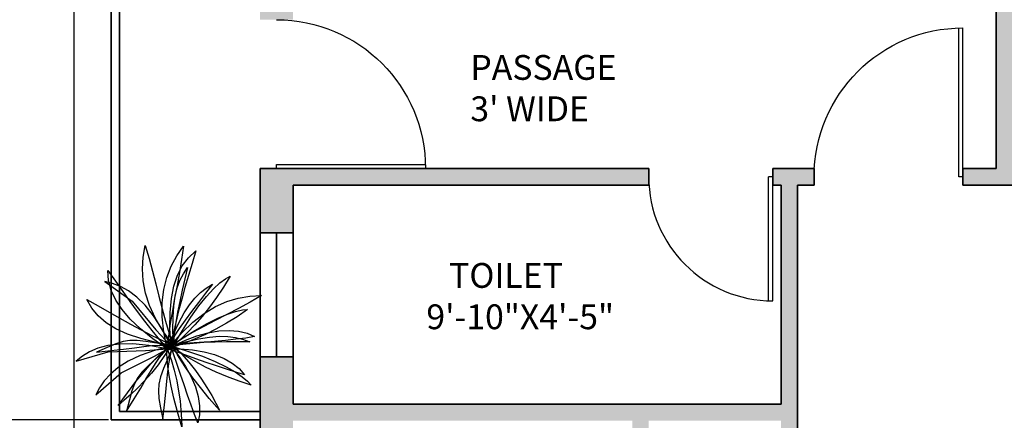
# Model space of a CAD drawing. Units: inches. Extents: x 1566 to 2546, y 1087 to 2705.
# Tile 19 of 27: x 2040 to 2278, y 1529 to 1625. Entities that reach past the tile are written whole.
import ezdxf

# ---------------------------------------------------------------- set-up
doc = ezdxf.new("R2010")
doc.units = ezdxf.units.IN
for name, color, linetype, lineweight in [('A-ANNO-DIMS', 2, 'Continuous', 18), ('A-AREA-IDEN', 7, 'Continuous', 18), ('A-DOOR', 4, 'Continuous', 25), ('A-WALL', 7, 'Continuous', 35), ('A-WALL-PATT', 8, 'Continuous', 13), ('L-PLNT', 94, 'Continuous', 18)]:
    doc.layers.add(name, color=color, linetype=linetype, lineweight=lineweight)
doc.layers.add('DIENHOA', color=3, linetype='Continuous')
doc.styles.get("Standard").update_dxf_attribs({"font": 'arial.ttf'})
doc.dimstyles.new('ISO-25', dxfattribs={"dimtxt": 2.5, "dimasz": 2.5, "dimexe": 1.25, "dimexo": 0.625, "dimtad": 1, "dimtxsty": 'Standard', "dimcen": 2.5, "dimadec": 0, "dimazin": 0, "dimtfac": 1, "dimtmove": 0, "dimatfit": 3, "dimfxl": 1, "dimarcsym": 0})

# ---------------------------------------------------------------- blocks, each defined once
blk = doc.blocks.new('*D3')
at = {"layer": 'A-ANNO-DIMS', "color": 0, "lineweight": -2, "transparency": 16777216}
for p, q in [((2061.66, 1784.43), (2052.02, 1784.43)), ((2053.27, 1781.93), (2053.27, 1162.93)), ((2061.66, 1160.43), (2052.02, 1160.43))]:
    blk.add_line(p, q, dxfattribs=at)
at = {"layer": 'A-ANNO-DIMS', "color": 0, "transparency": 16777216}
for points in [[(2052.85, 1781.93), (2053.69, 1781.93), (2053.27, 1784.43)], [(2052.85, 1162.93), (2053.69, 1162.93), (2053.27, 1160.43)]]:
    blk.add_solid(points, dxfattribs=at)
at = {"layer": 'Defpoints', "color": 0, "transparency": 16777216}
for p in [(2062.29, 1784.43), (2053.27, 1160.43), (2062.29, 1160.43)]:
    blk.add_point(p, dxfattribs=at)
at = {"layer": 'A-ANNO-DIMS', "color": 0, "transparency": 16777216, "insert": (2048.05, 1472.43), "char_height": 9, "attachment_point": 5, "rotation": 90}
blk.add_mtext("52'", dxfattribs=at)
blk = doc.blocks.new('d1')
for p, q in [((3297.32, 1596.93), (3297.32, 1632.93)), ((3298.32, 1596.93), (3298.32, 1632.93)), ((3297.32, 1596.93), (3298.32, 1596.93))]:
    blk.add_line(p, q)
at = {"ltscale": 0.3}
blk.add_arc((3297.32, 1596.93), 36, 0, 90, dxfattribs=at)
blk = doc.blocks.new('d2')
for p, q in [((3364.08, 1632.29), (3364.08, 1602.29)), ((3365.08, 1632.29), (3365.08, 1602.29)), ((3364.08, 1602.29), (3365.08, 1602.29))]:
    blk.add_line(p, q)
at = {"ltscale": 0.3}
blk.add_arc((3364.08, 1602.29), 30, 0, 90, dxfattribs=at)
blk = doc.blocks.new('Cay03_mb')
at = {"layer": 'DIENHOA'}
for p, q in [((118.6, 555.3), (166.2, 599.1)), ((166.2, 599.1), (142.2, 519.4)), ((48.6, 443.6), (79.5, 503.7)), ((79.5, 503.7), (118.6, 555.3)), ((142.2, 519.4), (119, 441.7)), ((25.5, 374.3), (48.6, 443.6)), ((119, 441.7), (96.7, 365.6)), ((-365.2, 390.3), (-414.4, 402.8)), ((-414.4, 402.8), (-240.2, 277.8)), ((-314.9, 371.3), (-365.2, 390.3)), ((-263.5, 343.5), (-314.9, 371.3)), ((-211.2, 304.6), (-263.5, 343.5)), ((9.9, 295.3), (25.5, 374.3)), ((96.7, 365.6), (75.6, 290.6)), ((-240.2, 277.8), (-88.4, 94.9)), ((-158, 252.3), (-211.2, 304.6)), ((-104.2, 184.4), (-158, 252.3)), ((1.6, 205.7), (9.9, 295.3)), ((75.6, 290.6), (55.7, 216.3)), ((290.6, 243.2), (363.4, 275.4)), ((363.4, 275.4), (436.8, 297.2)), ((436.8, 297.2), (511, 309.6)), ((511.8, 271.4), (437.6, 231.5)), ((511, 309.6), (585.9, 313.5)), ((585.9, 313.5), (511.8, 271.4)), ((0.2, 104.9), (1.6, 205.7)), ((55.7, 216.3), (37.3, 142.1)), ((147, 144.1), (218.5, 199.8)), ((218.5, 199.8), (290.6, 243.2)), ((363.7, 192.9), (290.2, 154.9)), ((437.6, 231.5), (363.7, 192.9)), ((-49.6, 98.5), (-104.2, 184.4)), ((37.3, 142.1), (20.5, 67.6)), ((75.9, 75.2), (147, 144.1)), ((290.2, 154.9), (217.4, 116.6)), ((-88.4, 94.9), (5.4, -7.8)), ((5.4, -7.8), (-49.6, 98.5)), ((5.4, -7.8), (0.2, 104.9)), ((5.4, -7.8), (75.9, 75.2)), ((20.5, 67.6), (5.4, -7.8)), ((145.5, 77.3), (74.7, 36.1)), ((217.4, 116.6), (145.5, 77.3)), ((-345, 5.4), (-399.6, -17.1)), ((-298.6, 20.1), (-345, 5.4)), ((-254.7, 27.4), (-298.6, 20.1)), ((-208, 27.8), (-254.7, 27.4)), ((-152.7, 21.7), (-208, 27.8)), ((-83.4, 9.7), (-152.7, 21.7)), ((5.4, -7.8), (-83.4, 9.7)), ((74.7, 36.1), (5.4, -7.8)), ((5.4, -7.8), (100.3, 18.4)), ((46.3, 0.9), (5.4, -7.8)), ((96.7, 7.5), (46.3, 0.9)), ((155, 12.2), (96.7, 7.5)), ((100.3, 18.4), (182.2, 37.2)), ((219.6, 15.4), (155, 12.2)), ((182.2, 37.2), (253, 48.9)), ((289, 17.4), (219.6, 15.4)), ((253, 48.9), (314.6, 54.1)), ((361.6, 18.5), (289, 17.4)), ((314.6, 54.1), (369.2, 53.3)), ((435.8, 18.9), (361.6, 18.5)), ((369.2, 53.3), (418.6, 46.8)), ((418.6, 46.8), (464.9, 35.2)), ((510, 19), (435.8, 18.9)), ((464.9, 35.2), (510, 19)), ((-399.6, -17.1), (-468, -47.9)), ((-468, -47.9), (-375.6, -37.8)), ((-375.6, -37.8), (-295.3, -27.9)), ((-295.3, -27.9), (-225.8, -18.9)), ((-225.8, -18.9), (-165.8, -11.3)), ((-165.8, -11.3), (-114, -5.7)), ((-114, -5.7), (-69, -2.9)), ((-79.8, -79.6), (-45.1, -46.3)), ((-69, -2.9), (-29.6, -3.4)), ((-45.1, -46.3), (-16.5, -22.4)), ((5.4, -7.8), (-33.2, -69.5)), ((-29.6, -3.4), (5.4, -7.8)), ((-16.5, -22.4), (5.4, -7.8)), ((5.4, -7.8), (56.8, -73.3)), ((25.9, -64.4), (5.4, -7.8)), ((5.4, -7.8), (112.8, -40.3)), ((53.5, -41.6), (5.4, -7.8)), ((107, -75.7), (53.5, -41.6)), ((112.8, -40.3), (207.5, -73.8)), ((-165.9, -174.1), (-120.2, -122.1)), ((-120.2, -122.1), (-79.8, -79.6)), ((-33.2, -69.5), (-74.6, -127.3)), ((47, -125.9), (25.9, -64.4)), ((56.8, -73.3), (100.4, -139.1)), ((165.5, -109.6), (107, -75.7)), ((228.7, -142.8), (165.5, -109.6)), ((207.5, -73.8), (289.5, -107.6)), ((289.5, -107.6), (359.3, -141.1)), ((-216.3, -235.6), (-165.9, -174.1)), ((-117.8, -181.1), (-162.1, -230.9)), ((-74.6, -127.3), (-117.8, -181.1)), ((68.7, -190.6), (47, -125.9)), ((100.4, -139.1), (135.9, -204.3)), ((296, -174.7), (228.7, -142.8)), ((367.1, -204.8), (296, -174.7)), ((359.3, -141.1), (416.9, -173.5)), ((416.9, -173.5), (462.6, -204.2)), ((-271, -306.6), (-216.3, -235.6)), ((-162.1, -230.9), (-206.3, -276.5)), ((90.8, -256.6), (68.7, -190.6)), ((135.9, -204.3), (162.8, -268.3)), ((441.6, -232.7), (367.1, -204.8)), ((518.9, -257.7), (441.6, -232.7)), ((462.6, -204.2), (496.5, -232.5)), ((496.5, -232.5), (518.9, -257.7)), ((-329.5, -387.1), (-271, -306.6)), ((-206.3, -276.5), (-249.6, -317.8)), ((113.1, -322.2), (90.8, -256.6)), ((162.8, -268.3), (181, -330.4)), ((-291, -354.7), (-329.5, -387.1)), ((-249.6, -317.8), (-291, -354.7)), ((135.4, -385.6), (113.1, -322.2)), ((181, -330.4), (190, -390)), ((157.6, -445), (135.4, -385.6)), ((190, -390), (189.6, -446.3)), ((179.5, -498.7), (157.6, -445)), ((189.6, -446.3), (179.5, -498.7))]:
    blk.add_line(p, q, dxfattribs=at)
for points in [[(23.7, -5.4), (-41, 82.2), (-91.8, 167.1), (-129.7, 249.5), (-155.6, 329.6), (-170.2, 407.8), (-174.7, 484.2), (-169.8, 559.3), (-156.5, 633.1)], [(-156.5, 633.1), (-132.5, 551.3), (-110.5, 470), (-89.8, 389.2), (-69.6, 309), (-49, 229.4), (-27.1, 150.4), (-3.2, 72.1), (23.7, -5.4)], [(-16.4, -26.7), (-38.3, 80), (-48.9, 178.3), (-48.7, 269), (-38.5, 352.6), (-19.1, 429.7), (9, 501), (44.9, 567.1), (87.9, 628.5)], [(87.9, 628.5), (75.5, 544.2), (61.3, 461.2), (46.1, 379.1), (30.8, 297.8), (16.1, 216.9), (2.9, 136), (-8.3, 54.9), (-16.4, -26.7)], [(-395.6, 473.7), (-347.5, 405.6), (-300.6, 339.5), (-254.3, 275.1), (-208.3, 212.3), (-161.9, 150.9), (-114.8, 90.7), (-66.5, 31.6), (-16.4, -26.7)], [(-16.4, -26.7), (-108.3, 38.6), (-186.9, 101.7), (-252.4, 163.5), (-305.1, 224.4), (-345.4, 285.2), (-373.7, 346.6), (-390.4, 409.2), (-395.6, 473.7)], [(23.7, -5.4), (19.8, 93), (20.3, 177), (25, 248.5), (34, 309.8), (47.3, 362.7), (64.9, 409.3), (86.8, 451.7), (112.9, 491.9)], [(112.9, 491.9), (96, 419.7), (79.5, 347.4), (63.9, 276.5), (50, 208.4), (38.4, 144.8), (29.7, 86.9), (24.6, 36.3), (23.7, -5.4)], [(273.2, 387.3), (227.6, 328.8), (182.3, 270.1), (138.4, 212.3), (97.2, 156.4), (60, 103.4), (27.8, 54.6), (1.9, 10.8), (-16.4, -26.7)], [(-16.4, -26.7), (21.4, 64.2), (57, 140.3), (91.4, 203.3), (125.2, 255.1), (159.5, 297.5), (195, 332.5), (232.7, 361.8), (273.2, 387.3)], [(384.3, 437.5), (342.2, 367.8), (298.1, 301.7), (252.6, 239.4), (206.1, 181.1), (159.4, 127.2), (113, 78), (67.6, 33.6), (23.7, -5.4)], [(23.7, -5.4), (79.9, 91.7), (134.1, 176.2), (185.8, 248.4), (234.3, 308.7), (279, 357.3), (319.3, 394.8), (354.6, 421.4), (384.3, 437.5)], [(-530.5, 289.7), (-458.3, 248.1), (-387.9, 207.8), (-318.9, 168.7), (-250.8, 131.1), (-182.9, 94.8), (-114.9, 59.9), (-46.2, 26.5), (23.7, -5.4)], [(23.7, -5.4), (-87.2, 15.2), (-185, 39.6), (-270.3, 68.2), (-343.7, 101.4), (-405.9, 139.7), (-457.3, 183.5), (-498.7, 233.4), (-530.5, 289.7)], [(496.7, 224), (429.4, 178.4), (361.6, 136.9), (294.1, 99.5), (227.5, 66.1), (162.4, 36.7), (99.7, 11.5), (39.8, -9.7), (-16.4, -26.7)], [(-16.4, -26.7), (75.4, 37.9), (160.1, 91.8), (237.3, 135.7), (306.6, 170), (367.6, 195.4), (419.9, 212.5), (463.1, 221.9), (496.7, 224)], [(23.7, -5.4), (99.3, 29.7), (173.2, 57.1), (244.8, 76.7), (313.3, 88.3), (377.9, 91.8), (437.9, 87), (492.7, 73.8), (541.4, 52)], [(-16.4, -26.7), (-134, -4.7), (-235.3, 5.3), (-322, 4.7), (-395.9, -5), (-458.7, -22.3), (-512.3, -45.7), (-558.2, -73.6), (-598.4, -104.7)], [(541.4, 52), (484.1, 42.9), (421.2, 34.8), (354.4, 27.6), (285.4, 20.9), (216.1, 14.5), (148.2, 8.1), (83.5, 1.6), (23.7, -5.4)], [(-598.4, -104.7), (-392.7, -44.4), (-155, -37.4), (-16.4, -26.7)], [(-471.9, -320.3), (-310.5, -179.3), (-97.7, -73.3), (23.7, -5.4)], [(23.7, -5.4), (-92.3, -34.8), (-188.4, -68.2), (-266.9, -105.1), (-329.9, -144.9), (-379.7, -187), (-418.5, -230.7), (-448.5, -275.3), (-471.9, -320.3)], [(-276.2, -424.4), (-227.3, -345.4), (-185.7, -276.1), (-150, -215.7), (-119.1, -163.8), (-91.5, -119.5), (-66, -82.3), (-41.4, -51.6), (-16.4, -26.7)], [(-16.4, -26.7), (-84.9, -86), (-137, -133.1), (-175.8, -173), (-204.3, -210), (-225.5, -249.1), (-242.5, -294.7), (-258.4, -351.6), (-276.2, -424.4)], [(23.7, -5.4), (-13.6, -87.9), (-41.1, -152.6), (-59.6, -205), (-69.9, -250.7), (-72.8, -295), (-69.2, -343.6), (-59.7, -401.9), (-45.3, -475.5)], [(-45.3, -475.5), (-34.1, -383.2), (-25.4, -302.8), (-18.3, -233.1), (-12, -172.9), (-5.6, -121.2), (2, -76.8), (11.4, -38.5), (23.7, -5.4)], [(76.2, -524.2), (48.8, -428.5), (26.6, -341.7), (9.2, -264.1), (-3.6, -196.1), (-12.3, -138), (-17.1, -90.2), (-18.3, -53), (-16.4, -26.7)], [(-16.4, -26.7), (66.9, -26.6), (145.6, -32.7), (218.8, -44.9), (285.8, -63.1), (345.9, -87.1), (398.4, -116.6), (442.6, -151.6), (477.6, -191.8)], [(477.6, -191.8), (421.8, -176), (361.3, -156.9), (297.6, -135.5), (232.2, -112.6), (166.6, -89.4), (102.3, -66.6), (40.8, -45.4), (-16.4, -26.7)], [(-16.4, -26.7), (8.5, -95.1), (28.5, -163.3), (44.3, -230.6), (56.3, -296.1), (65, -359), (70.9, -418.5), (74.5, -473.9), (76.2, -524.2)], [(316.5, -418.1), (251.4, -342.8), (194.8, -273.3), (146.5, -210.2), (106.3, -153.8), (74.1, -104.7), (49.7, -63.4), (32.9, -30.1), (23.7, -5.4)], [(23.7, -5.4), (74.9, -57.1), (121.8, -110.6), (164.3, -165), (202.7, -219.4), (237, -272.9), (267.3, -324.5), (293.7, -373.2), (316.5, -418.1)]]:
    blk.add_lwpolyline(points, dxfattribs=at)
blk = doc.blocks.new('*D91')
at = {"layer": 'A-ANNO-DIMS', "color": 0, "lineweight": -2, "transparency": 16777216}
for p, q in [((2061.66, 1784.43), (2016.94, 1784.43)), ((2018.19, 1781.93), (2018.19, 1531.18)), ((2061.66, 1528.68), (2016.94, 1528.68))]:
    blk.add_line(p, q, dxfattribs=at)
at = {"layer": 'A-ANNO-DIMS', "color": 0, "transparency": 16777216}
for points in [[(2017.77, 1781.93), (2018.6, 1781.93), (2018.19, 1784.43)], [(2017.77, 1531.18), (2018.6, 1531.18), (2018.19, 1528.68)]]:
    blk.add_solid(points, dxfattribs=at)
at = {"layer": 'Defpoints', "color": 0, "transparency": 16777216}
for p in [(2062.29, 1784.43), (2018.19, 1528.68), (2062.29, 1528.68)]:
    blk.add_point(p, dxfattribs=at)
at = {"layer": 'A-ANNO-DIMS', "color": 0, "transparency": 16777216, "insert": (2016.31, 1656.56), "char_height": 2.5, "attachment_point": 5, "rotation": 90}
blk.add_mtext('21\'-4"', dxfattribs=at)
blk = doc.blocks.new('*D92')
at = {"layer": 'A-ANNO-DIMS', "color": 0, "lineweight": -2, "transparency": 16777216}
for p, q in [((2061.66, 1528.68), (2016.94, 1528.68)), ((2018.19, 1526.18), (2018.19, 1477.15)), ((2061.66, 1474.65), (2016.94, 1474.65))]:
    blk.add_line(p, q, dxfattribs=at)
at = {"layer": 'A-ANNO-DIMS', "color": 0, "transparency": 16777216}
for points in [[(2017.77, 1526.18), (2018.6, 1526.18), (2018.19, 1528.68)], [(2017.77, 1477.15), (2018.6, 1477.15), (2018.19, 1474.65)]]:
    blk.add_solid(points, dxfattribs=at)
at = {"layer": 'Defpoints', "color": 0, "transparency": 16777216}
for p in [(2062.29, 1528.68), (2018.19, 1474.65), (2062.29, 1474.65)]:
    blk.add_point(p, dxfattribs=at)
at = {"layer": 'A-ANNO-DIMS', "color": 0, "transparency": 16777216, "insert": (2016.29, 1501.66), "char_height": 2.5, "attachment_point": 5, "rotation": 90}
blk.add_mtext('4\'-6"', dxfattribs=at)

msp = doc.modelspace()

# ---------------------------------------------------------------- hatches: boundary and pattern name
at = {"layer": 'A-WALL-PATT'}
h = msp.add_hatch(color=256, dxfattribs=at)
h.dxf.hatch_style = 1
h.paths.add_polyline_path([(2106.29, 1385.43), (2228.29, 1385.43), (2228.29, 1391.43), (2224.29, 1391.43), (2224.29, 1389.43), (2106.29, 1389.43), (2106.29, 1402.93), (2098.29, 1402.93), (2098.29, 1343.43), (2106.29, 1343.43), (2106.29, 1347.74)], flags=17)
h.paths.add_polyline_path([(2106.29, 1259.43), (2098.29, 1259.43), (2098.29, 1209.43), (2155.29, 1209.43), (2155.29, 1217.43), (2143.41, 1217.43), (2106.29, 1217.43)], flags=17)
h.paths.add_polyline_path([(2334.29, 1217.43), (2280.29, 1217.43), (2280.29, 1389.43), (2284.29, 1389.43), (2284.29, 1391.43), (2284.29, 1393.43), (2276.29, 1393.43), (2276.29, 1217.43), (2227.29, 1217.43), (2227.29, 1209.43), (2334.29, 1209.43)], flags=17)
h.paths.add_polyline_path([(2106.29, 1486.43), (2098.29, 1486.43), (2098.29, 1460.88), (2099.11, 1461.64), (2100.44, 1462.65), (2101.57, 1463.26), (2099.97, 1460.62), (2098.29, 1458.1), (2098.29, 1456.93), (2100.35, 1456.93), (2100.77, 1457.12), (2103.56, 1457.95), (2106.29, 1458.4), (2106.29, 1470.43), (2224.29, 1470.43), (2224.29, 1427.43), (2228.29, 1427.43), (2228.29, 1474.43), (2192.29, 1474.43), (2192.29, 1476.43), (2188.29, 1476.43), (2188.29, 1474.43), (2106.29, 1474.43)], flags=17)
h.paths.add_polyline_path([(2106.29, 1585.43), (2192.29, 1585.43), (2192.29, 1589.43), (2098.29, 1589.43), (2098.29, 1573.93), (2106.29, 1573.93)], flags=17)
h.paths.add_polyline_path([(2228.29, 1585.43), (2232.29, 1585.43), (2232.29, 1589.43), (2224.29, 1589.43), (2222.29, 1589.43), (2222.29, 1585.43), (2224.29, 1585.43), (2224.29, 1532.43), (2106.29, 1532.43), (2106.29, 1543.93), (2098.29, 1543.93), (2098.29, 1516.43), (2106.29, 1516.43), (2106.29, 1528.43), (2188.29, 1528.43), (2188.29, 1506.43), (2192.29, 1506.43), (2192.29, 1528.43), (2224.29, 1528.43), (2224.29, 1506.43), (2228.29, 1506.43)], flags=17)
h.paths.add_polyline_path([(2106.29, 1680.43), (2098.29, 1680.43), (2098.29, 1625.43), (2106.29, 1625.43)], flags=17)
h.paths.add_polyline_path([(2458.29, 1784.43), (2098.29, 1784.43), (2098.29, 1776.43), (2276.29, 1776.43), (2276.29, 1589.43), (2268.29, 1589.43), (2268.29, 1585.43), (2280.29, 1585.43), (2280.29, 1652.43), (2284.29, 1652.43), (2284.29, 1656.43), (2280.29, 1656.43), (2280.29, 1776.43), (2398.29, 1776.43), (2398.29, 1746.43), (2402.29, 1746.43), (2402.29, 1776.43), (2450.29, 1776.43), (2450.29, 1532.43), (2375.49, 1532.43), (2328.29, 1532.43), (2328.29, 1612.43), (2324.29, 1612.43), (2324.29, 1528.43), (2450.29, 1528.43), (2450.29, 1447.43), (2291.29, 1447.43), (2291.29, 1443.43), (2324.29, 1443.43), (2324.29, 1393.43), (2320.29, 1393.43), (2320.29, 1389.43), (2330.29, 1389.43), (2330.29, 1393.43), (2328.29, 1393.43), (2328.29, 1443.43), (2412.29, 1443.43), (2412.29, 1433.43), (2416.29, 1433.43), (2416.29, 1443.43), (2450.29, 1443.43), (2450.29, 1393.43), (2416.29, 1393.43), (2416.29, 1403.43), (2412.29, 1403.43), (2412.29, 1393.43), (2360.29, 1393.43), (2360.29, 1389.43), (2450.29, 1389.43), (2450.29, 1217.43), (2396.29, 1217.43), (2396.29, 1209.43), (2450.29, 1209.43), (2450.29, 1136.43), (2458.29, 1136.43)])

# ---------------------------------------------------------------- linework, layer by layer
at = {"layer": 'A-WALL'}
for p, q in [((2062.29, 1528.68), (2062.29, 1784.43)), ((2064.29, 1530.68), (2064.29, 1782.43)), ((2276.29, 1589.43), (2276.29, 1776.43)), ((2098.29, 1589.43), (2192.29, 1589.43)), ((2098.29, 1209.43), (2098.29, 1589.43)), ((2192.29, 1585.43), (2192.29, 1589.43)), ((2222.29, 1585.43), (2222.29, 1589.43)), ((2222.29, 1589.43), (2224.29, 1589.43)), ((2224.29, 1589.43), (2232.29, 1589.43)), ((2232.29, 1585.43), (2232.29, 1589.43)), ((2268.29, 1585.43), (2268.29, 1589.43)), ((2268.29, 1589.43), (2276.29, 1589.43)), ((2106.29, 1585.43), (2192.29, 1585.43)), ((2106.29, 1532.43), (2106.29, 1585.43)), ((2222.29, 1585.43), (2224.29, 1585.43)), ((2224.29, 1532.43), (2224.29, 1585.43)), ((2228.29, 1585.43), (2232.29, 1585.43)), ((2228.29, 1506.43), (2228.29, 1585.43)), ((2268.29, 1585.43), (2280.29, 1585.43)), ((2106.29, 1573.93), (2098.29, 1573.93)), ((2102.29, 1573.93), (2102.29, 1543.93)), ((2106.29, 1543.93), (2098.29, 1543.93)), ((2106.29, 1532.43), (2224.29, 1532.43)), ((2098.29, 1530.68), (2064.29, 1530.68)), ((2098.29, 1528.68), (2062.29, 1528.68))]:
    msp.add_line(p, q, dxfattribs=at)

# ---------------------------------------------------------------- block references
at = {"layer": 'A-DOOR', "xscale": -1, "rotation": 270}
msp.add_blockref('d1', (505.36, -1707.89), dxfattribs=at)
at = {"layer": 'A-DOOR', "xscale": -1}
msp.add_blockref('d1', (5565.61, -9.49), dxfattribs=at)
at = {"layer": 'A-DOOR', "rotation": 180}
msp.add_blockref('d2', (5586.37, 3189.73), dxfattribs=at)
at = {"layer": 'L-PLNT', "xscale": 0.0378941924884598, "yscale": 0.0378941924884598, "zscale": 0.0378941924884598}
msp.add_blockref('Cay03_mb', (2076.46, 1546.83), dxfattribs=at)

# ---------------------------------------------------------------- texts
at = {"layer": 'A-AREA-IDEN', "char_height": 6, "attachment_point": 1}
for s, insert in [("PASSAGE\\P3' WIDE", (2149.14, 1616.89)), ('   TOILET\\P9\'-10"X4\'-5"', (2138.5, 1566.59))]:
    msp.add_mtext_dynamic_manual_height_columns(s, width=111.7553, gutter_width=12.5, heights=[0], dxfattribs=dict(at, insert=insert))

# ---------------------------------------------------------------- dimensions: what is measured, and where the dimension line sits
at = {"layer": 'A-ANNO-DIMS'}
for base, p1, p2, override, picture, middle in [((2018.1868, 1528.6802), (2062.2895, 1784.433), (2062.2895, 1528.6802), {"dimdec": 1, "dimlfac": 1, "dimrnd": 0, "dimzin": 1, "dimdsep": 46, "dimlunit": 4, "dimfrac": 2}, '*D91', (2016.3067, 1656.5566)), ((2053.27, 1160.43), (2062.29, 1784.43), (2062.29, 1160.43), {"dimtxt": 9, "dimdec": 1, "dimlunit": 3, "dimclrd": 0, "dimclre": 0, "dimclrt": 0, "dimtdec": 1}, '*D3', (2048.05, 1472.43)), ((2018.19, 1474.65), (2062.29, 1528.68), (2062.29, 1474.65), {"dimdec": 1, "dimlfac": 1, "dimrnd": 0, "dimzin": 1, "dimdsep": 46, "dimlunit": 4, "dimfrac": 2}, '*D92', (2016.29, 1501.66))]:
    dim = msp.add_linear_dim(base=base, p1=p1, p2=p2, angle=90, dimstyle='ISO-25', override=override, dxfattribs=at)
    dim.commit()
    dim.dimension.update_dxf_attribs({"geometry": picture, "text_midpoint": middle})

doc.saveas('drawing.dxf')
